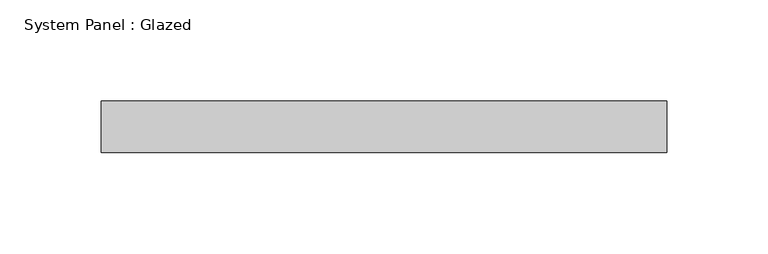
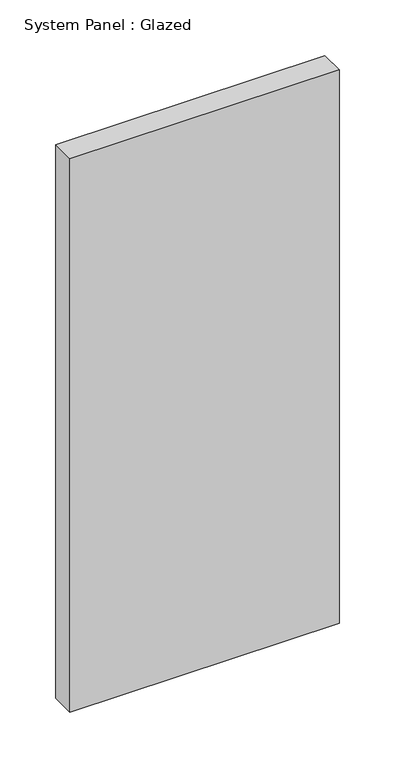
"""IFC4 building model written with IfcOpenShell, lengths in millimetres: plate geometry, System Panel : Glazed."""

from ifc_helpers import new_model, si_unit, origin, origin_with_axes, place, context, project, spatial, polyline, outline, extrude, source, transform, mapped, element, save


def system_panel_glazed_ef88186a(model_context):
    return source(origin(), model_context, "Body", "SweptSolid", [
        extrude(outline(polyline([(139.7, 19.05), (-139.7, 19.05), (-139.7, 44.45), (139.7, 44.45), (139.7, 19.05)])), origin_with_axes(), (0.0, 0.0, 1.0), 607.2495873),
    ])


if __name__ == "__main__":
    model = new_model("IFC4")
    model_context = context("Model", 3, world=origin())
    ifc_project = project(units=[si_unit("LENGTHUNIT", "METRE", prefix="MILLI")], contexts=[model_context])
    site = spatial("IfcSite", under=ifc_project)
    building = spatial("IfcBuilding", under=site)
    placement = place(None, origin())
    system_panel_glazed_shape = system_panel_glazed_ef88186a(model_context)
    element("IfcPlate", 1, ObjectType="System Panel : Glazed", at=placement, inside=building, context=model_context, shape_type="MappedRepresentation", body=[
        mapped(system_panel_glazed_shape, transform((0.0, 0.0, 0.0), x_axis=(1.0, 0.0, 0.0), y_axis=(0.0, 1.0, 0.0), z_axis=(0.0, 0.0, 1.0))),
    ])
    save(model, "model.ifc")

# Revit data of these elements
# Type "System Panel : Glazed"
#   Construction Type Id = "GSP4R"
#   Analytic Construction = "1/8 in Pilkington single glazing"
#   Visual Light Transmittance = 0.9
#   Solar Heat Gain Coefficient = 0.86
#   Heat Transfer Coefficient (U) = 1.18115 BTU/(h·ft²·°F)
#   Define Thermal Properties by = 1
# Element 1 (IfcPlate, "System Panel : Glazed")
#   Materials on its faces: "Glass"
# Materials
#   "Glass": class "Glass", colour RGB 0 128 192, transparency 0.75, Description = "Soda Lime Glass", Cost = 0
